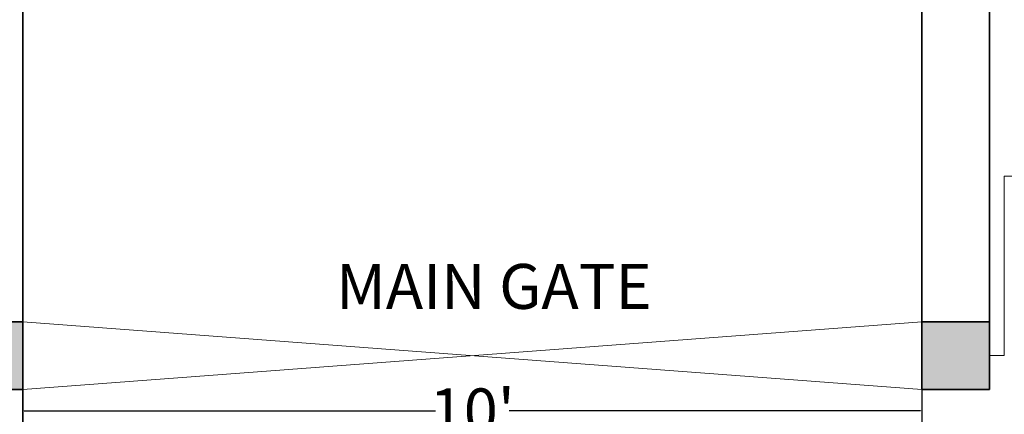
# Model space of a CAD drawing. Units: inches. Extents: x -36302355 to 648, y -221479757 to 75.
# Tile 4 of 37: x 154 to 285, y -583 to -531. Entities that reach past the tile are written whole.
import ezdxf

# ---------------------------------------------------------------- set-up
doc = ezdxf.new("R2010")
doc.units = ezdxf.units.IN
doc.header["$MEASUREMENT"] = 0
for name, color, linetype, lineweight in [('A-ANNO-DIMS', 2, 'Continuous', 18), ('A-ANNO-TEXT', 7, 'Continuous', 18), ('A-COLS', 7, 'Continuous', 35), ('A-COLS-PATT', 242, 'Continuous', 13), ('A-DOOR', 4, 'Continuous', 18), ('A-DOOR-GATE', 4, 'Continuous', 18), ('A-FLOR', 8, 'Continuous', 25), ('A-WALL', 7, 'Continuous', 35)]:
    doc.layers.add(name, color=color, linetype=linetype, lineweight=lineweight)
doc.styles.get("Standard").update_dxf_attribs({"font": 'arial.ttf'})
doc.dimstyles.get("Standard").update_dxf_attribs({"dimtxt": 0.18, "dimasz": 0.18, "dimexe": 0.18, "dimexo": 0.0625, "dimgap": 0.09, "dimtad": 0, "dimtih": 1, "dimtoh": 1, "dimdec": 0, "dimzin": 0, "dimdsep": 46, "dimlunit": 3, "dimtxsty": 'Standard', "dimcen": 0.09, "dimadec": 0, "dimazin": 0, "dimtfac": 1, "dimtdec": 0, "dimtofl": 0, "dimtmove": 0, "dimatfit": 3, "dimfxl": 1, "dimtolj": 1, "dimtzin": 0, "dimarcsym": 0})

# ---------------------------------------------------------------- blocks, each defined once
blk = doc.blocks.new('*D6')
at = {"layer": 'A-ANNO-DIMS', "color": 0, "lineweight": -2, "transparency": 16777216}
for p, q in [((154.2, -580.08), (154.2, -583.08)), ((274.2, -580.08), (274.2, -583.08)), ((154.38, -582.9), (209.3, -582.9)), ((274.02, -582.9), (219.1, -582.9))]:
    blk.add_line(p, q, dxfattribs=at)
at = {"layer": 'A-ANNO-DIMS', "color": 0, "transparency": 16777216}
for points in [[(154.38, -582.87), (154.38, -582.93), (154.2, -582.9)], [(274.02, -582.87), (274.02, -582.93), (274.2, -582.9)]]:
    blk.add_solid(points, dxfattribs=at)
at = {"layer": 'Defpoints', "color": 0, "transparency": 16777216}
for p in [(154.2, -580.02), (274.2, -580.02), (274.2, -582.9)]:
    blk.add_point(p, dxfattribs=at)
at = {"layer": 'A-ANNO-DIMS', "color": 0, "transparency": 16777216, "insert": (214.2, -582.9), "char_height": 6, "attachment_point": 5}
blk.add_mtext("\\A1;10'", dxfattribs=at)

msp = doc.modelspace()

# ---------------------------------------------------------------- hatches: boundary and pattern name
at = {"layer": 'A-COLS-PATT'}
h = msp.add_hatch(color=256, dxfattribs=at)
h.dxf.hatch_style = 1
h.paths.add_polyline_path([(145.2, 24.98), (145.2, 15.98), (154.2, 15.98), (154.2, 24.98)])
h.paths.add_polyline_path([(247.2, 15.98), (247.2, 24.98), (238.2, 24.98), (238.2, 15.98)])
h.paths.add_polyline_path([(387.64, 15.98), (395.7, 15.98), (395.7, 24.98), (387.64, 24.98)])
h.paths.add_polyline_path([(451.26, 24.98), (443.7, 24.98), (443.7, 15.98), (451.26, 15.98)])
h.paths.add_polyline_path([(596.2, 15.98), (605.2, 15.98), (605.2, 24.98), (596.2, 24.98)])
h.paths.add_polyline_path([(238.2, -122.02), (238.2, -131.02), (247.2, -131.02), (247.2, -122.02)])
h.paths.add_polyline_path([(395.7, -122.02), (387.46, -122.02), (387.46, -131.02), (395.7, -131.02)])
h.paths.add_polyline_path([(448.2, -131.02), (453.73, -131.02), (453.73, -122.02), (443.7, -122.02), (443.7, -131.02)])
h.paths.add_polyline_path([(596.2, -131.02), (605.2, -131.02), (605.2, -122.02), (596.2, -122.02)])
h.paths.add_polyline_path([(145.2, -176.97), (154.2, -176.97), (154.2, -167.02), (145.2, -167.02)])
h.paths.add_polyline_path([(314.2, -176.97), (323.2, -176.97), (323.2, -167.02), (314.2, -167.02)])
h.paths.add_polyline_path([(154.2, -314.02), (154.2, -309.52), (145.2, -309.52), (145.2, -314.02)])
h.paths.add_polyline_path([(314.2, -309.52), (314.2, -318.52), (323.2, -318.52), (323.2, -309.52)])
h.paths.add_polyline_path([(448.2, -277.02), (443.7, -277.02), (443.7, -286.02), (448.2, -286.02)])
h.paths.add_polyline_path([(283.2, -370.02), (274.2, -370.02), (274.2, -379.02), (283.2, -379.02), (283.2, -374.52)])
h.paths.add_polyline_path([(154.2, -370.02), (145.2, -370.02), (145.2, -379.02), (154.2, -379.02)])
h.paths.add_polyline_path([(443.2, -374.52), (443.2, -379.02), (452.2, -379.02), (452.2, -374.52)])
h.paths.add_polyline_path([(145.2, -580.02), (154.2, -580.02), (154.2, -571.02), (145.2, -571.02)])
h.paths.add_polyline_path([(274.2, -571.02), (274.2, -580.02), (283.2, -580.02), (283.2, -571.02)])
h.paths.add_polyline_path([(443.2, -580.02), (452.2, -580.02), (452.2, -571.02), (443.2, -571.02)])

# ---------------------------------------------------------------- linework, layer by layer
at = {"layer": 'A-COLS'}
for p, q in [((145.2, -571.02), (154.2, -571.02)), ((274.2, -571.02), (283.2, -571.02)), ((145.2, -580.02), (154.2, -580.02)), ((274.2, -580.02), (283.2, -580.02))]:
    msp.add_line(p, q, dxfattribs=at)
at = {"layer": 'A-DOOR'}
for p, q in [((285.2, -575.52), (285.2, -551.52)), ((283.2, -575.52), (285.2, -575.52))]:
    msp.add_line(p, q, dxfattribs=at)
msp.add_arc((285.2, -576.04), 24.52, 11.8123, 90, dxfattribs=at)
at = {"layer": 'A-DOOR-GATE'}
for p, q in [((154.2, -571.02), (274.2, -580.02)), ((274.2, -571.02), (154.2, -580.02))]:
    msp.add_line(p, q, dxfattribs=at)
at = {"layer": 'A-FLOR'}
msp.add_line((274.2, -580.02), (274.2, -651.02), dxfattribs=at)
at = {"layer": 'A-WALL'}
for p, q in [((154.2, -167.02), (154.2, -722.02)), ((274.2, -309.52), (274.2, -580.02)), ((283.2, -374.52), (283.2, -580.02))]:
    msp.add_line(p, q, dxfattribs=at)

# ---------------------------------------------------------------- texts
at = {"layer": 'A-ANNO-TEXT', "insert": (196.01, -563.27), "char_height": 6, "attachment_point": 1}
msp.add_mtext('MAIN GATE', dxfattribs=at)

# ---------------------------------------------------------------- dimensions: what is measured, and where the dimension line sits
at = {"layer": 'A-ANNO-DIMS'}
dim = msp.add_linear_dim(base=(274.2, -582.9), p1=(154.2, -580.02), p2=(274.2, -580.02), dimstyle='Standard', override={"dimtxt": 6, "dimclrd": 0, "dimclre": 0, "dimclrt": 0}, dxfattribs=at)
dim.commit()
dim.dimension.update_dxf_attribs({"geometry": '*D6', "text_midpoint": (214.2, -582.9)})

doc.saveas('drawing.dxf')
